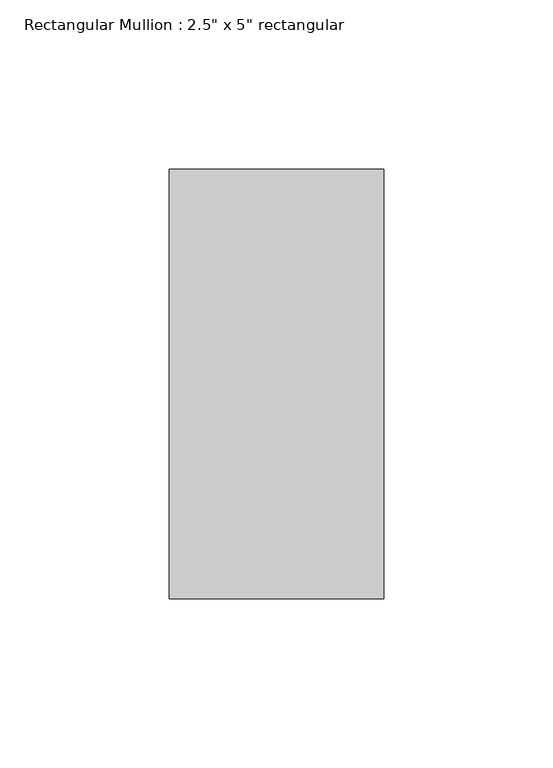
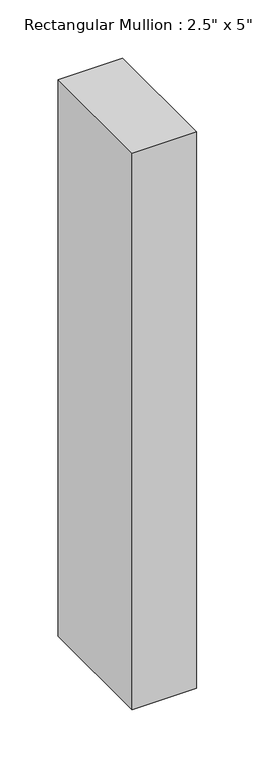
"""IFC4 building model written with IfcOpenShell, lengths in millimetres: member geometry."""

from ifc_helpers import new_model, si_unit, frame, origin, place, context, project, spatial, polyline, outline, extrude, source, transform, mapped, element, save


def member_9b8460a0(model_context):
    return source(origin(), model_context, "Body", "SweptSolid", [
        extrude(outline(polyline([(0.0, 63.5), (0.0, -63.5), (-63.5, -63.5), (-63.5, 63.5), (0.0, 63.5)])), frame((0.0, 0.0, -581.9828955), z_axis=(0.0, 0.0, 1.0), x_axis=(1.0, 0.0, 0.0)), (0.0, 0.0, 1.0), 581.9828955),
    ])


if __name__ == "__main__":
    model = new_model("IFC4")
    model_context = context("Model", 3, world=origin())
    ifc_project = project(units=[si_unit("LENGTHUNIT", "METRE", prefix="MILLI")], contexts=[model_context])
    site = spatial("IfcSite", under=ifc_project)
    building = spatial("IfcBuilding", under=site)
    placement = place(None, origin())
    member_shape = member_9b8460a0(model_context)
    element("IfcMember", 1, ObjectType="Rectangular Mullion : 2.5\" x 5\" rectangular", at=placement, inside=building, context=model_context, shape_type="MappedRepresentation", body=[
        mapped(member_shape, transform((0.0, 0.0, 0.0), x_axis=(1.0, 0.0, 0.0), y_axis=(0.0, 1.0, 0.0), z_axis=(0.0, 0.0, 1.0))),
    ])
    save(model, "model.ifc")

# Revit data of these elements
# Type "Rectangular Mullion : 2.5\" x 5\" rectangular"
#   built-in parameter 1007304 = 0.416667 (stored number, unit not read)
#   built-in parameter 1007301 = 0.104167 (stored number, unit not read)
#   built-in parameter 1007300 = 0.104167 (stored number, unit not read)
# Element 1 (IfcMember, "Rectangular Mullion : 2.5\" x 5\" rectangular")
#   Materials on its faces: "Aluminum"
# Materials
#   "Aluminum": class "Metal", colour RGB 247 247 247, transparency 0, Description = "Aluminum 6061", Cost = 0
